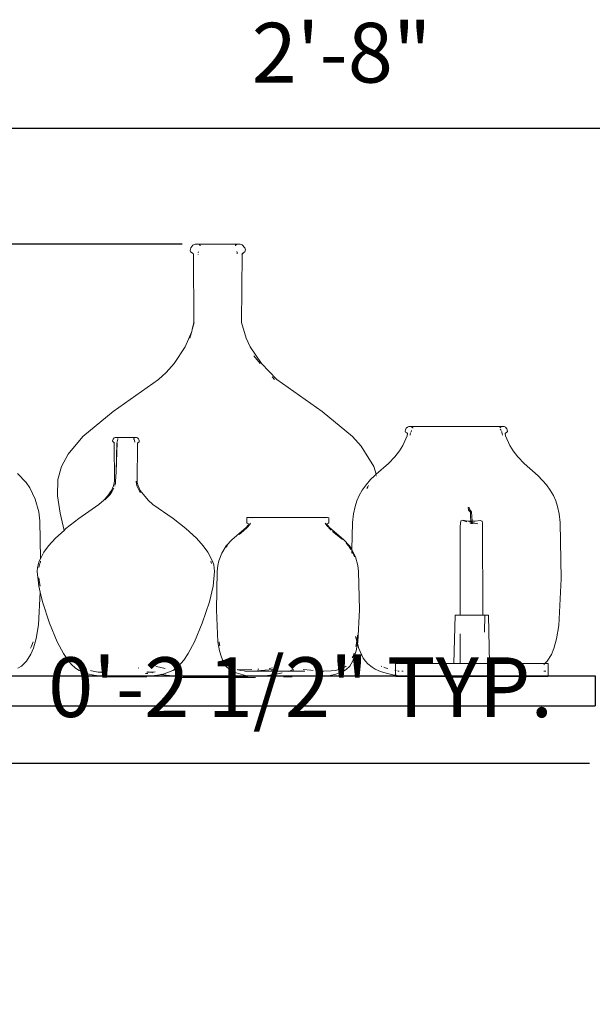
# Model space of a CAD drawing. Units: millimetres. Extents: x 7894 to 8038, y 6851 to 6951.
# Tile 47 of 49: x 7950.62 to 7960.21, y 6931.89 to 6948.36. Entities that reach past the tile are written whole.
import ezdxf

# ---------------------------------------------------------------- set-up
doc = ezdxf.new("R2010")
doc.units = ezdxf.units.MM
for name, color, linetype, lineweight in [('A-ANNO-DIMS', 2, 'Continuous', 18), ('A-FURN-ACCS', 8, 'Continuous', 13), ('A-FURN-SHLF', 7, 'Continuous', 30)]:
    doc.layers.add(name, color=color, linetype=linetype, lineweight=lineweight)
doc.styles.get("Standard").update_dxf_attribs({"font": 'arial.ttf'})
doc.dimstyles.new('ISO-25', dxfattribs={"dimtxt": 1, "dimasz": 1, "dimexe": 1.25, "dimexo": 0.625, "dimtad": 1, "dimdec": 0, "dimlunit": 4, "dimtxsty": 'Standard', "dimcen": 2.5, "dimclrt": 1, "dimadec": 0, "dimazin": 0, "dimtfac": 1, "dimtdec": 0, "dimtmove": 0, "dimatfit": 3, "dimfxl": 1, "dimarcsym": 0})

# ---------------------------------------------------------------- blocks, each defined once
blk = doc.blocks.new('FLOATING-SHELF-ELEV')
for p, q in [((0, 0.5), (17.304, 0.5)), ((0, 0.5), (0, 0)), ((17.304, 0.5), (17.304, 0)), ((0, 0), (17.304, 0))]:
    blk.add_line(p, q)
blk = doc.blocks.new('*D18')
at = {"layer": 'A-ANNO-DIMS', "color": 0, "lineweight": -2, "transparency": 16777216}
for p, q in [((7945.817, 6936.019), (7945.817, 6937.17)), ((7948.487, 6936.019), (7948.487, 6937.17)), ((7944.817, 6935.92), (7943.817, 6935.92)), ((7945.817, 6935.92), (7948.487, 6935.92)), ((7949.487, 6935.92), (7960.163, 6935.92))]:
    blk.add_line(p, q, dxfattribs=at)
at = {"layer": 'A-ANNO-DIMS', "color": 0, "transparency": 16777216}
for points in [[(7944.817, 6936.087), (7944.817, 6935.753), (7945.817, 6935.92)], [(7949.487, 6936.087), (7949.487, 6935.753), (7948.487, 6935.92)]]:
    blk.add_solid(points, dxfattribs=at)
at = {"layer": 'Defpoints', "color": 0, "transparency": 16777216}
for p in [(7948.487, 6935.92), (7945.817, 6935.394), (7948.487, 6935.394)]:
    blk.add_point(p, dxfattribs=at)
at = {"layer": 'A-ANNO-DIMS', "color": 1, "transparency": 16777216, "insert": (7955.325, 6937.062), "char_height": 1, "attachment_point": 5}
blk.add_mtext('0\'-2 1/2" TYP.', dxfattribs=at)
blk = doc.blocks.new('*D23')
at = {"layer": 'A-ANNO-DIMS', "color": 0, "lineweight": -2, "transparency": 16777216}
for p, q in [((7940.089, 6907.098), (7940.089, 6947.793)), ((7971.936, 6928.989), (7971.936, 6947.793)), ((7941.089, 6946.543), (7970.936, 6946.543))]:
    blk.add_line(p, q, dxfattribs=at)
at = {"layer": 'A-ANNO-DIMS', "color": 0, "transparency": 16777216}
for points in [[(7941.089, 6946.709), (7941.089, 6946.376), (7940.089, 6946.543)], [(7970.936, 6946.709), (7970.936, 6946.376), (7971.936, 6946.543)]]:
    blk.add_solid(points, dxfattribs=at)
at = {"layer": 'Defpoints', "color": 0, "transparency": 16777216}
for p in [(7971.936, 6946.543), (7971.936, 6928.364), (7940.089, 6906.473)]:
    blk.add_point(p, dxfattribs=at)
at = {"layer": 'A-ANNO-DIMS', "color": 1, "transparency": 16777216, "insert": (7956.012, 6947.678), "char_height": 1, "attachment_point": 5}
blk.add_mtext('2\'-8"', dxfattribs=at)
blk = doc.blocks.new('*D24')
at = {"layer": 'A-ANNO-DIMS', "color": 0, "lineweight": -2, "transparency": 16777216}
for p, q in [((7953.341, 6944.606), (7936.902, 6944.606)), ((7938.152, 6907.473), (7938.152, 6943.606)), ((7939.464, 6906.473), (7936.902, 6906.473))]:
    blk.add_line(p, q, dxfattribs=at)
at = {"layer": 'A-ANNO-DIMS', "color": 0, "transparency": 16777216}
for points in [[(7937.986, 6943.606), (7938.319, 6943.606), (7938.152, 6944.606)], [(7937.986, 6907.473), (7938.319, 6907.473), (7938.152, 6906.473)]]:
    blk.add_solid(points, dxfattribs=at)
at = {"layer": 'Defpoints', "color": 0, "transparency": 16777216}
for p in [(7938.152, 6944.606), (7953.966, 6944.606), (7940.089, 6906.473)]:
    blk.add_point(p, dxfattribs=at)
at = {"layer": 'A-ANNO-DIMS', "color": 1, "transparency": 16777216, "insert": (7937.016, 6925.539), "char_height": 1, "attachment_point": 5, "rotation": 90}
blk.add_mtext('3\'-2"', dxfattribs=at)

msp = doc.modelspace()

# ---------------------------------------------------------------- linework, layer by layer
at = {"layer": 'A-FURN-ACCS'}
for p, q in [((7953.485, 6944.54), (7953.475, 6944.498)), ((7953.485, 6944.54), (7953.519, 6944.587)), ((7953.56, 6944.606), (7953.519, 6944.587)), ((7953.56, 6944.606), (7953.565, 6944.606)), ((7953.565, 6944.606), (7953.632, 6944.596)), ((7953.565, 6944.606), (7953.724, 6944.606)), ((7953.632, 6944.596), (7953.641, 6944.58)), ((7953.641, 6944.58), (7953.641, 6944.576)), ((7953.772, 6944.606), (7953.724, 6944.606)), ((7953.813, 6944.606), (7953.772, 6944.606)), ((7953.966, 6944.606), (7953.813, 6944.606)), ((7954.008, 6944.606), (7953.966, 6944.606)), ((7954.31, 6944.606), (7954.008, 6944.606)), ((7954.257, 6944.604), (7954.231, 6944.599)), ((7954.231, 6944.599), (7954.252, 6944.601)), ((7954.245, 6944.598), (7954.234, 6944.58)), ((7954.234, 6944.58), (7954.234, 6944.577)), ((7954.252, 6944.601), (7954.245, 6944.598)), ((7954.252, 6944.601), (7954.31, 6944.606)), ((7954.257, 6944.604), (7954.252, 6944.601)), ((7954.348, 6944.592), (7954.31, 6944.606)), ((7954.391, 6944.54), (7954.348, 6944.592)), ((7954.4, 6944.507), (7954.391, 6944.54)), ((7953.483, 6944.473), (7953.475, 6944.498)), ((7953.483, 6944.473), (7953.524, 6944.445)), ((7953.53, 6944.429), (7953.524, 6944.445)), ((7953.538, 6943.295), (7953.53, 6944.429)), ((7953.611, 6944.465), (7953.61, 6944.458)), ((7953.61, 6944.435), (7953.61, 6944.431)), ((7953.614, 6944.473), (7953.611, 6944.465)), ((7954.255, 6944.48), (7954.26, 6944.465)), ((7954.264, 6944.465), (7954.259, 6944.48)), ((7954.265, 6944.441), (7954.264, 6944.465)), ((7954.345, 6944.431), (7954.337, 6943.295)), ((7954.361, 6944.455), (7954.339, 6944.431)), ((7954.339, 6944.431), (7954.354, 6944.445)), ((7954.345, 6944.431), (7954.354, 6944.445)), ((7954.354, 6944.445), (7954.373, 6944.463)), ((7954.354, 6944.445), (7954.361, 6944.455)), ((7954.382, 6944.47), (7954.361, 6944.455)), ((7954.361, 6944.455), (7954.373, 6944.463)), ((7954.373, 6944.463), (7954.392, 6944.473)), ((7954.373, 6944.463), (7954.382, 6944.47)), ((7954.392, 6944.473), (7954.4, 6944.507)), ((7953.51, 6943.174), (7953.538, 6943.295)), ((7953.544, 6943.295), (7953.51, 6943.174)), ((7954.337, 6943.295), (7954.414, 6943.031)), ((7953.393, 6942.885), (7953.501, 6943.145)), ((7953.501, 6943.145), (7953.469, 6943.031)), ((7953.51, 6943.174), (7953.501, 6943.145)), ((7953.208, 6942.606), (7953.393, 6942.885)), ((7954.482, 6942.885), (7954.414, 6943.031)), ((7954.668, 6942.606), (7954.482, 6942.885)), ((7954.529, 6942.754), (7954.529, 6942.755)), ((7954.645, 6942.606), (7954.542, 6942.738)), ((7953.075, 6942.459), (7953.208, 6942.606)), ((7954.929, 6942.342), (7954.668, 6942.606)), ((7952.946, 6942.342), (7953.075, 6942.459)), ((7954.888, 6942.342), (7954.846, 6942.382)), ((7952.187, 6941.803), (7952.946, 6942.342)), ((7955.688, 6941.803), (7954.929, 6942.342)), ((7952.187, 6941.803), (7951.68, 6941.384)), ((7956.195, 6941.384), (7955.688, 6941.803)), ((7957.038, 6941.234), (7957.11, 6941.399)), ((7957.078, 6941.474), (7957.081, 6941.497)), ((7957.078, 6941.474), (7957.084, 6941.46)), ((7957.081, 6941.497), (7957.094, 6941.524)), ((7957.105, 6941.449), (7957.084, 6941.46)), ((7957.094, 6941.524), (7957.113, 6941.542)), ((7957.115, 6941.434), (7957.105, 6941.449)), ((7957.11, 6941.399), (7957.115, 6941.434)), ((7957.113, 6941.542), (7957.136, 6941.552)), ((7957.136, 6941.552), (7957.185, 6941.548)), ((7957.136, 6941.552), (7957.724, 6941.552)), ((7957.163, 6941.431), (7957.159, 6941.407)), ((7957.17, 6941.452), (7957.163, 6941.431)), ((7957.182, 6941.489), (7957.175, 6941.466)), ((7957.185, 6941.548), (7957.204, 6941.533)), ((7957.204, 6941.533), (7957.205, 6941.524)), ((7957.73, 6941.552), (7957.724, 6941.552)), ((7957.73, 6941.552), (7958.703, 6941.552)), ((7958.661, 6941.549), (7958.692, 6941.55)), ((7958.672, 6941.544), (7958.663, 6941.533)), ((7958.669, 6941.507), (7958.681, 6941.497)), ((7958.692, 6941.55), (7958.672, 6941.544)), ((7958.681, 6941.497), (7958.684, 6941.489)), ((7958.691, 6941.468), (7958.693, 6941.463)), ((7958.703, 6941.552), (7958.692, 6941.55)), ((7958.695, 6941.457), (7958.704, 6941.432)), ((7958.705, 6941.552), (7958.703, 6941.552)), ((7958.704, 6941.432), (7958.708, 6941.407)), ((7958.705, 6941.552), (7958.733, 6941.552)), ((7958.755, 6941.541), (7958.733, 6941.552)), ((7958.752, 6941.434), (7958.756, 6941.442)), ((7958.757, 6941.399), (7958.752, 6941.434)), ((7958.778, 6941.515), (7958.755, 6941.541)), ((7958.756, 6941.442), (7958.781, 6941.459)), ((7958.829, 6941.234), (7958.757, 6941.399)), ((7958.786, 6941.497), (7958.778, 6941.515)), ((7958.781, 6941.459), (7958.788, 6941.47)), ((7958.788, 6941.47), (7958.786, 6941.497)), ((7951.434, 6941.093), (7951.68, 6941.384)), ((7952.183, 6941.342), (7952.175, 6941.311)), ((7952.175, 6941.311), (7952.179, 6941.298)), ((7952.189, 6941.292), (7952.179, 6941.298)), ((7952.181, 6941.3), (7952.189, 6941.292)), ((7952.203, 6941.363), (7952.183, 6941.342)), ((7952.189, 6941.292), (7952.201, 6941.281)), ((7952.201, 6941.281), (7952.205, 6941.274)), ((7952.201, 6941.281), (7952.208, 6941.274)), ((7952.221, 6941.371), (7952.203, 6941.363)), ((7952.205, 6941.274), (7952.209, 6940.637)), ((7952.238, 6941.371), (7952.221, 6941.371)), ((7952.233, 6940.792), (7952.251, 6941.285)), ((7952.233, 6940.792), (7952.249, 6941.285)), ((7952.251, 6941.37), (7952.238, 6941.371)), ((7952.25, 6941.294), (7952.265, 6941.341)), ((7952.251, 6941.37), (7952.252, 6941.371)), ((7952.251, 6941.37), (7952.262, 6941.365)), ((7952.252, 6941.371), (7952.546, 6941.371)), ((7952.265, 6941.352), (7952.262, 6941.365)), ((7952.531, 6941.357), (7952.532, 6941.359)), ((7952.532, 6941.354), (7952.531, 6941.357)), ((7952.532, 6941.354), (7952.531, 6941.338)), ((7952.533, 6941.365), (7952.532, 6941.36)), ((7952.537, 6941.336), (7952.532, 6941.354)), ((7952.533, 6941.36), (7952.536, 6941.366)), ((7952.547, 6941.37), (7952.536, 6941.366)), ((7952.547, 6941.295), (7952.538, 6941.333)), ((7952.546, 6941.371), (7952.547, 6941.37)), ((7952.559, 6941.371), (7952.547, 6941.37)), ((7952.548, 6941.289), (7952.547, 6941.295)), ((7952.548, 6941.274), (7952.548, 6941.277)), ((7952.576, 6941.371), (7952.559, 6941.371)), ((7952.592, 6941.363), (7952.576, 6941.371)), ((7952.593, 6941.273), (7952.59, 6940.616)), ((7952.592, 6941.363), (7952.61, 6941.348)), ((7952.593, 6941.273), (7952.596, 6941.282)), ((7952.596, 6941.282), (7952.619, 6941.298)), ((7952.62, 6941.327), (7952.61, 6941.348)), ((7952.619, 6941.298), (7952.623, 6941.308)), ((7952.62, 6941.327), (7952.623, 6941.308)), ((7956.342, 6941.225), (7956.195, 6941.384)), ((7956.981, 6941.147), (7957.038, 6941.234)), ((7958.885, 6941.147), (7958.829, 6941.234)), ((7951.321, 6940.886), (7951.434, 6941.093)), ((7956.342, 6941.225), (7956.554, 6940.886)), ((7956.902, 6941.046), (7956.981, 6941.147)), ((7958.965, 6941.046), (7958.885, 6941.147)), ((7956.591, 6940.756), (7956.797, 6940.934)), ((7956.797, 6940.934), (7956.902, 6941.046)), ((7959.07, 6940.934), (7958.965, 6941.046)), ((7959.305, 6940.73), (7959.07, 6940.934)), ((7950.584, 6940.769), (7950.727, 6940.616)), ((7951.321, 6940.886), (7951.259, 6940.668)), ((7952.233, 6940.792), (7952.227, 6940.633)), ((7956.591, 6940.756), (7956.554, 6940.886)), ((7956.561, 6940.73), (7956.591, 6940.756)), ((7950.727, 6940.616), (7950.79, 6940.526)), ((7951.259, 6940.668), (7951.255, 6940.394)), ((7952.209, 6940.637), (7952.193, 6940.561)), ((7952.226, 6940.613), (7952.216, 6940.572)), ((7952.225, 6940.595), (7952.226, 6940.613)), ((7952.227, 6940.616), (7952.226, 6940.613)), ((7952.227, 6940.633), (7952.227, 6940.616)), ((7952.57, 6940.626), (7952.569, 6940.637)), ((7952.584, 6940.563), (7952.57, 6940.626)), ((7952.59, 6940.616), (7952.604, 6940.561)), ((7956.421, 6940.579), (7956.358, 6940.49)), ((7956.421, 6940.579), (7956.496, 6940.666)), ((7956.496, 6940.666), (7956.561, 6940.73)), ((7956.6, 6940.725), (7956.598, 6940.73)), ((7959.446, 6940.579), (7959.305, 6940.73)), ((7959.508, 6940.49), (7959.446, 6940.579)), ((7950.79, 6940.526), (7950.881, 6940.34)), ((7952.045, 6940.327), (7952.134, 6940.416)), ((7952.091, 6940.387), (7952.158, 6940.483)), ((7952.171, 6940.473), (7952.134, 6940.416)), ((7952.158, 6940.483), (7952.193, 6940.561)), ((7952.195, 6940.524), (7952.171, 6940.473)), ((7952.213, 6940.563), (7952.211, 6940.557)), ((7952.627, 6940.473), (7952.584, 6940.563)), ((7952.604, 6940.561), (7952.639, 6940.483)), ((7952.646, 6940.447), (7952.627, 6940.473)), ((7952.639, 6940.483), (7952.769, 6940.32)), ((7956.358, 6940.49), (7956.308, 6940.399)), ((7956.45, 6940.546), (7956.433, 6940.518)), ((7956.464, 6940.564), (7956.45, 6940.546)), ((7959.559, 6940.399), (7959.508, 6940.49)), ((7950.881, 6940.34), (7950.938, 6940.124)), ((7951.295, 6940.102), (7951.255, 6940.394)), ((7951.948, 6940.25), (7951.609, 6940.013)), ((7952.029, 6940.32), (7951.948, 6940.25)), ((7952.091, 6940.387), (7952.029, 6940.32)), ((7952.849, 6940.25), (7952.769, 6940.32)), ((7953.188, 6940.013), (7952.849, 6940.25)), ((7956.238, 6940.212), (7956.268, 6940.307)), ((7956.268, 6940.307), (7956.308, 6940.399)), ((7959.599, 6940.307), (7959.559, 6940.399)), ((7959.629, 6940.212), (7959.599, 6940.307)), ((7950.938, 6940.124), (7950.957, 6939.975)), ((7951.362, 6939.815), (7951.295, 6940.102)), ((7956.193, 6939.946), (7956.211, 6940.093)), ((7956.211, 6940.093), (7956.238, 6940.212)), ((7958.151, 6940.198), (7958.131, 6940.196)), ((7958.136, 6940.156), (7958.131, 6940.196)), ((7958.171, 6940.117), (7958.136, 6940.156)), ((7958.156, 6940.17), (7958.151, 6940.198)), ((7958.189, 6940.126), (7958.156, 6940.17)), ((7958.172, 6940.048), (7958.171, 6940.117)), ((7958.189, 6940.126), (7958.199, 6939.968)), ((7959.656, 6940.093), (7959.629, 6940.212)), ((7959.674, 6939.946), (7959.656, 6940.093)), ((7950.957, 6939.975), (7950.969, 6939.341)), ((7951.394, 6939.844), (7951.609, 6940.013)), ((7953.403, 6939.844), (7953.188, 6940.013)), ((7954.429, 6940.029), (7954.426, 6940.023)), ((7954.427, 6939.943), (7954.426, 6940.023)), ((7954.427, 6939.943), (7954.432, 6939.934)), ((7954.436, 6940.032), (7954.429, 6940.029)), ((7954.432, 6939.934), (7954.454, 6939.926)), ((7954.471, 6939.91), (7954.435, 6939.867)), ((7954.458, 6940.032), (7954.436, 6940.032)), ((7954.436, 6940.032), (7954.492, 6940.028)), ((7954.457, 6939.916), (7954.449, 6939.9)), ((7954.454, 6939.926), (7954.457, 6939.916)), ((7954.463, 6940.033), (7954.458, 6940.032)), ((7954.463, 6940.033), (7954.536, 6940.033)), ((7954.471, 6939.91), (7954.487, 6939.938)), ((7954.492, 6940.028), (7954.496, 6940.026)), ((7954.492, 6940.028), (7954.511, 6940.027)), ((7954.511, 6940.027), (7954.512, 6940.027)), ((7954.632, 6940.032), (7954.536, 6940.033)), ((7954.632, 6940.032), (7954.776, 6940.032)), ((7954.776, 6940.032), (7954.936, 6940.033)), ((7954.939, 6940.033), (7954.936, 6940.033)), ((7954.939, 6940.033), (7954.942, 6940.033)), ((7954.942, 6940.033), (7955.109, 6940.032)), ((7955.289, 6940.032), (7955.109, 6940.032)), ((7955.443, 6940.033), (7955.289, 6940.032)), ((7955.45, 6940.033), (7955.443, 6940.033)), ((7955.45, 6940.033), (7955.585, 6940.033)), ((7955.695, 6940.032), (7955.585, 6940.033)), ((7955.763, 6940.032), (7955.695, 6940.032)), ((7955.727, 6940.026), (7955.763, 6940.032)), ((7955.781, 6939.877), (7955.736, 6939.934)), ((7955.765, 6940.032), (7955.763, 6940.032)), ((7955.765, 6940.032), (7955.778, 6940.033)), ((7955.768, 6939.925), (7955.766, 6939.92)), ((7955.766, 6939.92), (7955.77, 6939.907)), ((7955.79, 6939.933), (7955.768, 6939.925)), ((7955.778, 6940.033), (7955.796, 6940.027)), ((7955.796, 6939.943), (7955.79, 6939.933)), ((7955.796, 6940.027), (7955.796, 6939.943)), ((7956.184, 6939.497), (7956.193, 6939.946)), ((7958, 6939.88), (7958.011, 6939.973)), ((7958.036, 6939.985), (7958.011, 6939.973)), ((7958.129, 6939.968), (7958.036, 6939.985)), ((7958.11, 6939.958), (7958.045, 6939.979)), ((7958.045, 6939.979), (7958.129, 6939.968)), ((7958.129, 6939.968), (7958.174, 6939.968)), ((7958.175, 6939.956), (7958.129, 6939.968)), ((7958.175, 6939.938), (7958.162, 6939.942)), ((7958.174, 6939.968), (7958.172, 6940.048)), ((7958.175, 6939.956), (7958.174, 6939.968)), ((7958.174, 6939.968), (7958.199, 6939.968)), ((7958.201, 6939.949), (7958.175, 6939.956)), ((7958.175, 6939.952), (7958.175, 6939.954)), ((7958.175, 6939.938), (7958.175, 6939.946)), ((7958.188, 6939.934), (7958.175, 6939.938)), ((7958.175, 6939.929), (7958.175, 6939.938)), ((7958.192, 6939.928), (7958.175, 6939.929)), ((7958.188, 6939.934), (7958.202, 6939.933)), ((7958.192, 6939.928), (7958.202, 6939.928)), ((7958.199, 6939.968), (7958.201, 6939.949)), ((7958.199, 6939.968), (7958.247, 6939.968)), ((7958.295, 6939.925), (7958.201, 6939.949)), ((7958.201, 6939.946), (7958.201, 6939.937)), ((7958.202, 6939.933), (7958.202, 6939.928)), ((7958.202, 6939.933), (7958.25, 6939.928)), ((7958.247, 6939.968), (7958.331, 6939.98)), ((7958.331, 6939.98), (7958.365, 6939.967)), ((7958.373, 6939.937), (7958.365, 6939.967)), ((7958.373, 6939.937), (7958.375, 6938.398)), ((7959.691, 6939.003), (7959.674, 6939.946)), ((7951.218, 6939.682), (7951.362, 6939.815)), ((7951.362, 6939.815), (7951.394, 6939.844)), ((7953.579, 6939.682), (7953.403, 6939.844)), ((7954.408, 6939.856), (7954.177, 6939.66)), ((7954.295, 6939.745), (7954.371, 6939.806)), ((7954.371, 6939.806), (7954.435, 6939.867)), ((7954.449, 6939.9), (7954.408, 6939.856)), ((7955.77, 6939.907), (7955.816, 6939.856)), ((7955.838, 6939.82), (7955.791, 6939.865)), ((7955.816, 6939.856), (7956.046, 6939.66)), ((7956.024, 6939.666), (7955.862, 6939.798)), ((7958, 6938.398), (7958, 6939.88)), ((7951.104, 6939.555), (7951.218, 6939.682)), ((7953.693, 6939.555), (7953.579, 6939.682)), ((7954.177, 6939.66), (7954.081, 6939.557)), ((7956.031, 6939.66), (7956.024, 6939.666)), ((7956.046, 6939.66), (7956.142, 6939.557)), ((7956.131, 6939.55), (7956.091, 6939.599)), ((7951.026, 6939.449), (7950.969, 6939.341)), ((7951.104, 6939.555), (7951.026, 6939.449)), ((7953.772, 6939.449), (7953.693, 6939.555)), ((7953.772, 6939.449), (7953.85, 6939.3)), ((7954.005, 6939.435), (7953.957, 6939.308)), ((7954.081, 6939.557), (7954.005, 6939.435)), ((7954.079, 6939.532), (7954.092, 6939.55)), ((7954.092, 6939.55), (7954.098, 6939.557)), ((7956.164, 6939.497), (7956.131, 6939.55)), ((7956.142, 6939.557), (7956.184, 6939.497)), ((7956.183, 6939.466), (7956.184, 6939.497)), ((7956.184, 6939.464), (7956.183, 6939.466)), ((7956.183, 6939.431), (7956.184, 6939.464)), ((7956.184, 6939.497), (7956.246, 6939.372)), ((7956.207, 6939.426), (7956.184, 6939.464)), ((7956.228, 6939.372), (7956.207, 6939.426)), ((7950.919, 6939.195), (7950.947, 6939.3)), ((7950.942, 6939.195), (7950.958, 6939.262)), ((7950.969, 6939.341), (7950.947, 6939.3)), ((7950.97, 6939.285), (7950.958, 6939.262)), ((7950.97, 6939.3), (7950.971, 6939.288)), ((7950.971, 6939.288), (7950.97, 6939.286)), ((7950.97, 6939.286), (7950.97, 6939.285)), ((7953.822, 6939.3), (7953.834, 6939.262)), ((7953.87, 6939.237), (7953.85, 6939.3)), ((7953.957, 6939.308), (7953.939, 6939.226)), ((7956.246, 6939.372), (7956.285, 6939.226)), ((7950.913, 6939.126), (7950.919, 6939.195)), ((7950.913, 6939.126), (7950.939, 6938.882)), ((7953.884, 6939.126), (7953.859, 6938.882)), ((7953.884, 6939.126), (7953.87, 6939.237)), ((7953.926, 6939.126), (7953.914, 6938.484)), ((7953.939, 6939.226), (7953.926, 6939.126)), ((7956.285, 6939.226), (7956.297, 6939.126)), ((7956.297, 6939.126), (7956.309, 6938.484)), ((7950.94, 6939.023), (7950.95, 6938.943)), ((7950.95, 6938.943), (7950.964, 6938.882)), ((7959.652, 6938.222), (7959.691, 6939.003)), ((7950.962, 6938.78), (7950.935, 6938.232)), ((7950.962, 6938.78), (7950.939, 6938.882)), ((7951, 6938.621), (7950.962, 6938.78)), ((7953.859, 6938.882), (7953.798, 6938.621)), ((7951.118, 6938.26), (7951, 6938.621)), ((7953.798, 6938.621), (7953.679, 6938.26)), ((7953.914, 6938.484), (7953.941, 6937.952)), ((7956.309, 6938.484), (7956.282, 6937.952)), ((7957.894, 6937.587), (7957.912, 6938.395)), ((7957.912, 6938.395), (7957.916, 6938.398)), ((7957.916, 6938.398), (7957.94, 6938.398)), ((7957.94, 6938.398), (7957.941, 6938.398)), ((7957.941, 6938.398), (7957.952, 6938.398)), ((7957.952, 6938.398), (7957.954, 6938.398)), ((7957.954, 6938.398), (7957.955, 6938.398)), ((7957.955, 6938.398), (7957.963, 6938.398)), ((7957.963, 6938.398), (7957.966, 6938.398)), ((7957.966, 6938.398), (7957.969, 6938.398)), ((7957.969, 6938.398), (7957.97, 6938.398)), ((7957.97, 6938.398), (7957.972, 6938.398)), ((7957.972, 6938.398), (7957.974, 6938.398)), ((7957.976, 6938.398), (7957.974, 6938.398)), ((7957.974, 6938.398), (7957.974, 6938.395)), ((7957.976, 6938.398), (7957.978, 6938.398)), ((7957.978, 6938.398), (7957.981, 6938.398)), ((7957.986, 6938.398), (7957.981, 6938.398)), ((7957.988, 6938.398), (7957.986, 6938.398)), ((7957.988, 6938.398), (7957.993, 6938.398)), ((7957.993, 6938.398), (7957.995, 6938.398)), ((7957.995, 6938.398), (7957.995, 6938.398)), ((7957.995, 6938.398), (7958, 6938.398)), ((7958, 6938.395), (7958, 6938.398)), ((7958.007, 6938.398), (7958, 6938.398)), ((7958.007, 6938.398), (7958.016, 6938.398)), ((7958.046, 6938.398), (7958.016, 6938.398)), ((7958.051, 6938.398), (7958.046, 6938.398)), ((7958.051, 6938.398), (7958.075, 6938.398)), ((7958.075, 6938.398), (7958.081, 6938.398)), ((7958.081, 6938.398), (7958.119, 6938.398)), ((7958.126, 6938.398), (7958.119, 6938.398)), ((7958.126, 6938.398), (7958.14, 6938.398)), ((7958.18, 6938.398), (7958.14, 6938.398)), ((7958.18, 6938.398), (7958.182, 6938.398)), ((7958.182, 6938.398), (7958.225, 6938.398)), ((7958.234, 6938.398), (7958.225, 6938.398)), ((7958.234, 6938.398), (7958.26, 6938.398)), ((7958.26, 6938.398), (7958.266, 6938.398)), ((7958.281, 6938.398), (7958.266, 6938.398)), ((7958.283, 6938.398), (7958.281, 6938.398)), ((7958.286, 6938.398), (7958.283, 6938.398)), ((7958.286, 6938.398), (7958.287, 6938.398)), ((7958.287, 6938.398), (7958.288, 6938.398)), ((7958.288, 6938.398), (7958.303, 6938.398)), ((7958.308, 6938.398), (7958.303, 6938.398)), ((7958.32, 6938.398), (7958.308, 6938.398)), ((7958.32, 6938.398), (7958.322, 6938.398)), ((7958.322, 6938.398), (7958.354, 6938.398)), ((7958.358, 6938.398), (7958.354, 6938.398)), ((7958.358, 6938.398), (7958.369, 6938.398)), ((7958.372, 6938.398), (7958.369, 6938.398)), ((7958.375, 6938.398), (7958.372, 6938.398)), ((7958.375, 6938.398), (7958.375, 6938.395)), ((7958.378, 6938.398), (7958.375, 6938.398)), ((7958.375, 6938.398), (7958.375, 6938.398)), ((7958.379, 6938.398), (7958.378, 6938.398)), ((7958.379, 6938.398), (7958.385, 6938.398)), ((7958.387, 6938.398), (7958.385, 6938.398)), ((7958.396, 6938.398), (7958.387, 6938.398)), ((7958.398, 6938.398), (7958.396, 6938.398)), ((7958.398, 6938.398), (7958.403, 6938.398)), ((7958.409, 6938.398), (7958.403, 6938.398)), ((7958.409, 6938.398), (7958.405, 6938.112)), ((7958.411, 6938.398), (7958.409, 6938.398)), ((7958.413, 6938.398), (7958.411, 6938.398)), ((7958.413, 6938.398), (7958.424, 6938.398)), ((7958.424, 6938.398), (7958.427, 6938.398)), ((7958.427, 6938.398), (7958.43, 6938.398)), ((7958.43, 6938.398), (7958.439, 6938.398)), ((7958.439, 6938.398), (7958.441, 6938.398)), ((7958.441, 6938.398), (7958.442, 6938.398)), ((7958.442, 6938.398), (7958.447, 6938.398)), ((7958.447, 6938.398), (7958.468, 6938.398)), ((7958.471, 6938.395), (7958.468, 6938.398)), ((7958.49, 6937.587), (7958.471, 6938.395)), ((7950.935, 6938.232), (7950.895, 6938.006)), ((7951.118, 6938.26), (7951.249, 6937.952)), ((7953.548, 6937.952), (7953.679, 6938.26)), ((7959.612, 6937.999), (7959.652, 6938.222)), ((7950.819, 6937.876), (7950.843, 6937.948)), ((7950.895, 6938.006), (7950.85, 6937.846)), ((7951.356, 6937.753), (7951.249, 6937.952)), ((7953.548, 6937.952), (7953.442, 6937.753)), ((7953.941, 6937.952), (7953.968, 6937.8)), ((7953.967, 6937.9), (7953.96, 6937.952)), ((7956.254, 6937.999), (7956.247, 6938.039)), ((7956.265, 6937.962), (7956.254, 6937.999)), ((7956.256, 6937.9), (7956.265, 6937.962)), ((7956.265, 6937.962), (7956.279, 6938.062)), ((7956.276, 6937.921), (7956.265, 6937.962)), ((7956.282, 6937.952), (7956.276, 6937.921)), ((7958, 6937.587), (7958, 6938.082)), ((7959.568, 6937.841), (7959.612, 6937.999)), ((7950.803, 6937.846), (7950.819, 6937.876)), ((7950.85, 6937.846), (7950.807, 6937.742)), ((7953.973, 6937.881), (7953.967, 6937.9)), ((7953.968, 6937.8), (7953.999, 6937.693)), ((7956.255, 6937.8), (7956.225, 6937.693)), ((7956.249, 6937.873), (7956.256, 6937.9)), ((7956.276, 6937.921), (7956.255, 6937.8)), ((7956.299, 6937.841), (7956.276, 6937.921)), ((7956.374, 6937.677), (7956.299, 6937.841)), ((7959.525, 6937.738), (7959.568, 6937.841)), ((7950.736, 6937.627), (7950.649, 6937.544)), ((7950.807, 6937.742), (7950.736, 6937.627)), ((7951.356, 6937.753), (7951.428, 6937.644)), ((7951.481, 6937.577), (7951.428, 6937.644)), ((7953.281, 6937.541), (7953.37, 6937.644)), ((7953.37, 6937.644), (7953.442, 6937.753)), ((7953.999, 6937.693), (7954.027, 6937.622)), ((7954.027, 6937.622), (7954.075, 6937.545)), ((7956.196, 6937.622), (7956.148, 6937.545)), ((7956.189, 6937.684), (7956.204, 6937.713)), ((7956.225, 6937.693), (7956.196, 6937.622)), ((7956.204, 6937.713), (7956.22, 6937.761)), ((7956.411, 6937.624), (7956.374, 6937.677)), ((7956.452, 6937.58), (7956.411, 6937.624)), ((7959.416, 6937.587), (7959.456, 6937.624)), ((7959.456, 6937.624), (7959.525, 6937.738)), ((7950.649, 6937.544), (7950.59, 6937.507)), ((7951.553, 6937.51), (7951.481, 6937.577)), ((7951.614, 6937.471), (7951.553, 6937.51)), ((7951.756, 6937.415), (7951.614, 6937.471)), ((7951.68, 6937.516), (7951.656, 6937.532)), ((7951.713, 6937.504), (7951.68, 6937.516)), ((7951.822, 6937.465), (7951.808, 6937.47)), ((7951.934, 6937.444), (7951.822, 6937.465)), ((7952.01, 6937.441), (7951.934, 6937.444)), ((7952.603, 6937.515), (7952.616, 6937.51)), ((7952.801, 6937.442), (7952.752, 6937.44)), ((7952.765, 6937.451), (7952.774, 6937.448)), ((7952.774, 6937.448), (7952.801, 6937.442)), ((7952.863, 6937.444), (7952.801, 6937.442)), ((7952.801, 6937.442), (7952.811, 6937.44)), ((7952.863, 6937.444), (7952.888, 6937.45)), ((7952.912, 6937.538), (7952.9, 6937.541)), ((7952.912, 6937.538), (7953.055, 6937.506)), ((7953.183, 6937.471), (7953.042, 6937.415)), ((7953.183, 6937.471), (7953.244, 6937.51)), ((7953.281, 6937.541), (7953.244, 6937.51)), ((7954.075, 6937.545), (7954.134, 6937.489)), ((7954.103, 6937.577), (7954.094, 6937.584)), ((7954.134, 6937.489), (7954.186, 6937.456)), ((7954.186, 6937.456), (7954.245, 6937.43)), ((7954.287, 6937.481), (7954.26, 6937.488)), ((7954.27, 6937.48), (7954.287, 6937.481)), ((7954.287, 6937.481), (7954.507, 6937.489)), ((7954.319, 6937.472), (7954.287, 6937.481)), ((7954.388, 6937.463), (7954.319, 6937.472)), ((7954.492, 6937.457), (7954.386, 6937.46)), ((7954.532, 6937.46), (7954.388, 6937.463)), ((7954.406, 6937.457), (7954.492, 6937.457)), ((7954.602, 6937.457), (7954.492, 6937.457)), ((7954.728, 6937.475), (7954.532, 6937.46)), ((7954.532, 6937.46), (7955.132, 6937.46)), ((7954.609, 6937.493), (7954.623, 6937.493)), ((7954.728, 6937.475), (7954.729, 6937.475)), ((7954.858, 6937.489), (7954.729, 6937.475)), ((7954.801, 6937.502), (7954.855, 6937.515)), ((7954.922, 6937.489), (7954.833, 6937.475)), ((7954.862, 6937.489), (7954.86, 6937.489)), ((7954.922, 6937.489), (7954.927, 6937.489)), ((7955.132, 6937.46), (7955.123, 6937.456)), ((7955.191, 6937.483), (7955.132, 6937.46)), ((7955.396, 6937.46), (7955.132, 6937.46)), ((7955.191, 6937.483), (7955.178, 6937.489)), ((7955.183, 6937.489), (7955.191, 6937.483)), ((7955.191, 6937.483), (7955.193, 6937.484)), ((7955.206, 6937.489), (7955.193, 6937.484)), ((7955.193, 6937.484), (7955.212, 6937.475)), ((7955.367, 6937.489), (7955.494, 6937.475)), ((7955.494, 6937.475), (7955.533, 6937.472)), ((7955.628, 6937.466), (7955.713, 6937.46)), ((7955.713, 6937.46), (7955.643, 6937.46)), ((7955.713, 6937.46), (7955.835, 6937.463)), ((7955.835, 6937.463), (7955.904, 6937.472)), ((7955.904, 6937.472), (7955.969, 6937.487)), ((7955.969, 6937.487), (7955.974, 6937.489)), ((7956.037, 6937.456), (7955.978, 6937.43)), ((7956.034, 6937.517), (7956.08, 6937.538)), ((7956.089, 6937.489), (7956.037, 6937.456)), ((7956.08, 6937.538), (7956.088, 6937.545)), ((7956.148, 6937.545), (7956.089, 6937.489)), ((7956.522, 6937.525), (7956.452, 6937.58)), ((7956.575, 6937.494), (7956.522, 6937.525)), ((7956.662, 6937.455), (7956.575, 6937.494)), ((7956.756, 6937.425), (7956.662, 6937.455)), ((7956.673, 6937.542), (7956.685, 6937.537)), ((7956.718, 6937.524), (7956.744, 6937.513)), ((7956.744, 6937.513), (7956.785, 6937.502)), ((7956.903, 6937.474), (7956.915, 6937.472)), ((7956.915, 6937.472), (7956.915, 6937.587)), ((7957.894, 6937.587), (7956.915, 6937.587)), ((7956.915, 6937.472), (7956.923, 6937.47)), ((7956.915, 6937.393), (7956.915, 6937.472)), ((7956.955, 6937.464), (7956.974, 6937.461)), ((7956.955, 6937.458), (7956.961, 6937.458)), ((7956.961, 6937.458), (7956.978, 6937.457)), ((7956.974, 6937.461), (7956.978, 6937.46)), ((7957.023, 6937.459), (7957.041, 6937.458)), ((7957.023, 6937.457), (7957.041, 6937.457)), ((7958, 6937.587), (7957.894, 6937.587)), ((7958, 6937.587), (7958.49, 6937.587)), ((7959.399, 6937.587), (7958.49, 6937.587)), ((7959.399, 6937.57), (7959.416, 6937.587)), ((7959.399, 6937.587), (7959.416, 6937.587)), ((7959.423, 6937.458), (7959.399, 6937.457)), ((7959.421, 6937.587), (7959.416, 6937.587)), ((7959.428, 6937.587), (7959.421, 6937.587)), ((7959.434, 6937.458), (7959.423, 6937.458)), ((7959.428, 6937.587), (7959.469, 6937.587)), ((7959.469, 6937.38), (7959.469, 6937.587)), ((7951.861, 6937.392), (7951.756, 6937.415)), ((7952, 6937.374), (7951.861, 6937.392)), ((7952, 6937.374), (7952.252, 6937.373)), ((7952.107, 6937.363), (7952.048, 6937.363)), ((7952.252, 6937.373), (7952.107, 6937.363)), ((7952.731, 6937.363), (7952.107, 6937.363)), ((7952.252, 6937.373), (7952.301, 6937.373)), ((7952.301, 6937.373), (7952.34, 6937.373)), ((7952.34, 6937.373), (7952.36, 6937.373)), ((7952.361, 6937.373), (7952.36, 6937.373)), ((7952.409, 6937.373), (7952.433, 6937.373)), ((7952.476, 6937.373), (7952.433, 6937.373)), ((7952.476, 6937.373), (7952.497, 6937.373)), ((7952.497, 6937.373), (7952.778, 6937.374)), ((7952.667, 6937.369), (7952.497, 6937.373)), ((7952.731, 6937.363), (7952.667, 6937.369)), ((7952.725, 6937.42), (7952.747, 6937.42)), ((7952.729, 6937.421), (7952.747, 6937.42)), ((7952.749, 6937.363), (7952.731, 6937.363)), ((7952.766, 6937.42), (7952.747, 6937.42)), ((7952.927, 6937.392), (7952.778, 6937.374)), ((7952.836, 6937.435), (7952.843, 6937.433)), ((7952.987, 6937.404), (7952.927, 6937.392)), ((7952.982, 6937.405), (7952.987, 6937.404)), ((7953.042, 6937.415), (7952.987, 6937.404)), ((7952.987, 6937.404), (7953.216, 6937.373)), ((7953.668, 6937.37), (7953.216, 6937.373)), ((7953.304, 6937.352), (7953.315, 6937.352)), ((7953.315, 6937.352), (7953.397, 6937.363)), ((7953.315, 6937.352), (7954.539, 6937.352)), ((7953.668, 6937.37), (7953.397, 6937.363)), ((7953.539, 6937.373), (7953.457, 6937.373)), ((7953.588, 6937.372), (7953.539, 6937.373)), ((7953.588, 6937.372), (7953.668, 6937.37)), ((7953.67, 6937.372), (7953.588, 6937.372)), ((7953.668, 6937.37), (7953.828, 6937.371)), ((7953.828, 6937.371), (7953.67, 6937.372)), ((7953.828, 6937.371), (7953.839, 6937.371)), ((7953.839, 6937.371), (7953.909, 6937.371)), ((7953.909, 6937.371), (7953.92, 6937.37)), ((7953.934, 6937.371), (7953.92, 6937.37)), ((7953.946, 6937.371), (7953.934, 6937.371)), ((7953.956, 6937.371), (7953.946, 6937.371)), ((7953.962, 6937.371), (7953.956, 6937.371)), ((7953.971, 6937.371), (7953.962, 6937.371)), ((7953.987, 6937.371), (7953.971, 6937.371)), ((7954.022, 6937.371), (7953.987, 6937.371)), ((7954.022, 6937.371), (7954.049, 6937.371)), ((7954.255, 6937.372), (7954.049, 6937.371)), ((7954.202, 6937.37), (7954.049, 6937.371)), ((7954.202, 6937.37), (7954.255, 6937.372)), ((7954.202, 6937.37), (7954.344, 6937.363)), ((7954.245, 6937.43), (7954.402, 6937.389)), ((7954.478, 6937.373), (7954.255, 6937.372)), ((7954.344, 6937.363), (7954.539, 6937.352)), ((7954.402, 6937.389), (7954.544, 6937.375)), ((7954.478, 6937.373), (7954.541, 6937.373)), ((7954.572, 6937.352), (7954.539, 6937.352)), ((7954.544, 6937.375), (7954.541, 6937.373)), ((7954.544, 6937.375), (7954.605, 6937.375)), ((7954.605, 6937.375), (7954.646, 6937.373)), ((7954.654, 6937.374), (7954.646, 6937.373)), ((7954.654, 6937.374), (7955.023, 6937.373)), ((7954.893, 6937.405), (7954.77, 6937.389)), ((7955.015, 6937.43), (7954.893, 6937.405)), ((7955.023, 6937.373), (7955.084, 6937.37)), ((7955.039, 6937.365), (7955.048, 6937.365)), ((7955.084, 6937.37), (7955.048, 6937.365)), ((7955.048, 6937.365), (7955.184, 6937.365)), ((7955.104, 6937.37), (7955.084, 6937.37)), ((7955.086, 6937.373), (7955.104, 6937.37)), ((7955.104, 6937.37), (7955.107, 6937.371)), ((7955.107, 6937.371), (7955.112, 6937.37)), ((7955.112, 6937.37), (7955.117, 6937.37)), ((7955.117, 6937.37), (7955.118, 6937.37)), ((7955.213, 6937.373), (7955.118, 6937.37)), ((7955.118, 6937.37), (7955.184, 6937.365)), ((7955.677, 6937.375), (7955.213, 6937.373)), ((7955.677, 6937.375), (7955.698, 6937.375)), ((7955.821, 6937.389), (7955.698, 6937.375)), ((7955.821, 6937.389), (7955.913, 6937.409)), ((7955.978, 6937.43), (7955.913, 6937.409)), ((7956.892, 6937.395), (7956.756, 6937.425)), ((7956.915, 6937.393), (7956.892, 6937.395)), ((7956.915, 6937.38), (7956.915, 6937.393)), ((7956.929, 6937.391), (7956.915, 6937.393)), ((7956.924, 6937.369), (7956.915, 6937.38)), ((7957.244, 6937.369), (7956.924, 6937.369)), ((7956.992, 6937.384), (7956.955, 6937.388)), ((7957.043, 6937.377), (7957.019, 6937.38)), ((7957.176, 6937.374), (7957.186, 6937.374)), ((7957.189, 6937.374), (7957.186, 6937.374)), ((7957.22, 6937.374), (7957.189, 6937.374)), ((7957.223, 6937.374), (7957.22, 6937.374)), ((7957.255, 6937.369), (7957.244, 6937.369)), ((7957.26, 6937.369), (7957.255, 6937.369)), ((7957.26, 6937.369), (7957.427, 6937.369)), ((7957.405, 6937.373), (7957.346, 6937.373)), ((7957.427, 6937.369), (7957.348, 6937.369)), ((7957.407, 6937.373), (7957.405, 6937.373)), ((7957.436, 6937.37), (7957.427, 6937.369)), ((7957.445, 6937.369), (7957.436, 6937.37)), ((7957.445, 6937.369), (7957.899, 6937.369)), ((7957.827, 6937.36), (7957.903, 6937.367)), ((7957.827, 6937.36), (7958.036, 6937.36)), ((7957.903, 6937.367), (7957.899, 6937.369)), ((7957.903, 6937.367), (7957.924, 6937.369)), ((7957.945, 6937.367), (7957.924, 6937.369)), ((7957.953, 6937.369), (7957.945, 6937.367)), ((7957.953, 6937.369), (7957.975, 6937.367)), ((7957.975, 6937.367), (7957.985, 6937.369)), ((7958.036, 6937.36), (7957.975, 6937.367)), ((7957.985, 6937.369), (7959.139, 6937.369)), ((7959.139, 6937.369), (7959.217, 6937.369)), ((7959.274, 6937.369), (7959.217, 6937.369)), ((7959.274, 6937.369), (7959.284, 6937.369)), ((7959.284, 6937.369), (7959.285, 6937.369)), ((7959.284, 6937.369), (7959.286, 6937.369)), ((7959.286, 6937.369), (7959.333, 6937.369)), ((7959.333, 6937.369), (7959.342, 6937.369)), ((7959.342, 6937.369), (7959.343, 6937.369)), ((7959.343, 6937.369), (7959.382, 6937.369)), ((7959.382, 6937.369), (7959.409, 6937.369)), ((7959.409, 6937.369), (7959.419, 6937.369)), ((7959.425, 6937.369), (7959.419, 6937.369)), ((7959.459, 6937.369), (7959.425, 6937.369)), ((7959.459, 6937.369), (7959.469, 6937.38))]:
    msp.add_line(p, q, dxfattribs=at)

# ---------------------------------------------------------------- block references
at = {"layer": 'A-FURN-SHLF'}
msp.add_blockref('FLOATING-SHELF-ELEV', (7942.957, 6936.88), dxfattribs=at)

# ---------------------------------------------------------------- dimensions: what is measured, and where the dimension line sits
at = {"layer": 'A-ANNO-DIMS'}
dim = msp.add_linear_dim(base=(7971.936, 6946.543), p1=(7940.089, 6906.473), p2=(7971.936, 6928.364), dimstyle='ISO-25', override={"dimdec": 1, "dimlfac": 1, "dimrnd": 0, "dimzin": 1, "dimdsep": 46, "dimlunit": 4, "dimfrac": 2}, dxfattribs=at)
dim.commit()
dim.dimension.update_dxf_attribs({"geometry": '*D23', "text_midpoint": (7956.012, 6947.678)})
dim = msp.add_linear_dim(base=(7938.152, 6944.606), p1=(7940.089, 6906.473), p2=(7953.966, 6944.606), angle=90, dimstyle='ISO-25', override={"dimdec": 1, "dimlfac": 1, "dimrnd": 0, "dimzin": 1, "dimdsep": 46, "dimlunit": 4, "dimfrac": 2}, dxfattribs=at)
dim.commit()
dim.dimension.update_dxf_attribs({"geometry": '*D24', "text_midpoint": (7937.016, 6925.539)})
dim = msp.add_linear_dim(base=(7948.487, 6935.92), p1=(7945.817, 6935.394), p2=(7948.487, 6935.394), text='<> TYP.', dimstyle='ISO-25', override={"dimdec": 1, "dimlfac": 1, "dimrnd": 0, "dimzin": 1, "dimdsep": 46, "dimlunit": 4, "dimfrac": 2}, dxfattribs=at)
dim.commit()
dim.dimension.update_dxf_attribs({"geometry": '*D18', "text_midpoint": (7955.325, 6937.062)})

doc.saveas('drawing.dxf')
